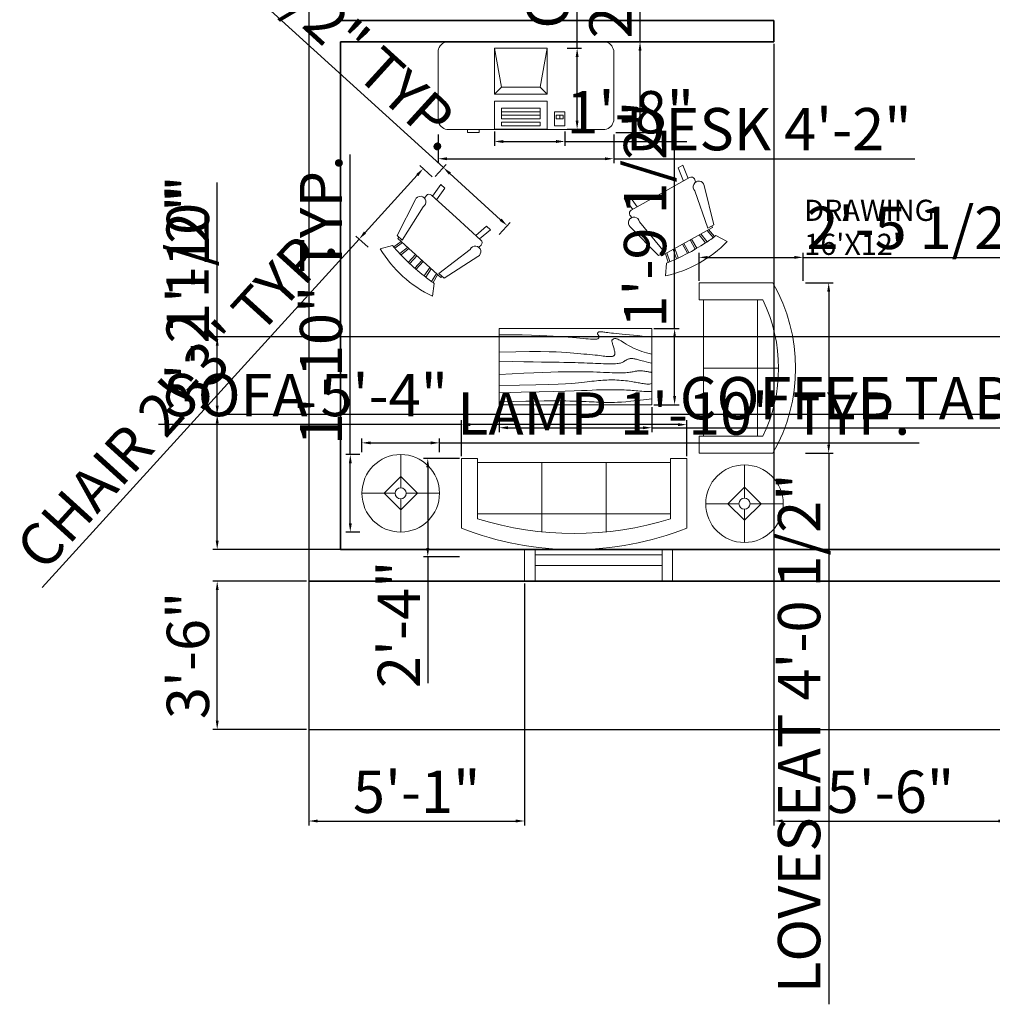
# Model space of a CAD drawing. Units: inches. Extents: x 2021 to 2692, y 429 to 1061.
# Tile 1 of 5: x 2086 to 2362, y 429 to 708. Entities that reach past the tile are written whole.
import ezdxf

# ---------------------------------------------------------------- set-up
doc = ezdxf.new("R2010")
doc.units = ezdxf.units.IN
for name, color, linetype, lineweight in [('A-ANNO-DIMS', 2, 'Continuous', 18), ('A-AREA-IDEN', 7, 'Continuous', 18), ('A-EQPM', 8, 'Continuous', 13), ('A-FURN', 8, 'Continuous', 13), ('A-GLAZ', 4, 'Continuous', 18), ('A-WALL', 7, 'Continuous', 35), ('C-PROP', 3, 'Continuous', 25)]:
    doc.layers.add(name, color=color, linetype=linetype, lineweight=lineweight)
doc.styles.get("Standard").update_dxf_attribs({"font": 'arial.ttf'})
doc.dimstyles.new('ISO-25', dxfattribs={"dimtxt": 12, "dimasz": 2.5, "dimexe": 1.25, "dimexo": 0.625, "dimtad": 1, "dimdec": 0, "dimlunit": 3, "dimtxsty": 'Standard', "dimcen": 2.5, "dimadec": 0, "dimazin": 0, "dimtfac": 1, "dimtdec": 0, "dimtmove": 0, "dimatfit": 3, "dimfxl": 1, "dimarcsym": 0})

# ---------------------------------------------------------------- blocks, each defined once
blk = doc.blocks.new('Desk - 30 x 60 in.')
for p, q in [((-26.999995, 0), (26.999995, 0)), ((-29.999995, -27), (-29.999995, -3)), ((29.999995, -3), (29.999995, -27)), ((26.999995, -30), (-26.999995, -30)), ((-20.000005, -30), (-20.000005, -31)), ((-16.000005, -31), (-16.000005, -30)), ((15.999995, -31), (15.999995, -30)), ((19.999995, -30), (19.999995, -31)), ((-20.000005, -31), (-16.000005, -31)), ((19.999995, -31), (15.999995, -31))]:
    blk.add_line(p, q)
for centre, start, end in [((-26.499995, -3.5), 98.1301, 171.8699), ((26.499995, -3.5), 8.130102, 81.8699), ((-26.499995, -26.5), 188.1301, 261.8699), ((26.499995, -26.5), 278.1301, 351.8699)]:
    blk.add_arc(centre, 3.535534, start, end)
blk = doc.blocks.new('Chair - Rocking')
for p, q in [((-8, -4.5), (-10, -1.5)), ((8, -4.5), (10, -1.5)), ((-7.5, -4.5), (-7, -7)), ((-6.5, -7), (-7.02225, -4.43)), ((-4.5, -7), (-4.96674, -4.19951)), ((-4, -7), (-4.40532, -4.16272)), ((-1.5, -4.05012), (-1.5, -7)), ((-1, -7), (-1, -4.05012)), ((1, -7), (1, -4.04655)), ((1.5, -4.05012), (1.5, -7)), ((4, -7), (4.40187, -4.18694)), ((4.5, -7), (4.96761, -4.19437)), ((6.5, -7), (7, -4.4057)), ((7.5, -4.5), (7, -7)), ((-9, -7.5), (-12, -18.49999)), ((-7, -7.5), (-9, -7.5)), ((-9, -18.49999), (-7, -7.5)), ((-8.23428, -6.99939), (-8.3093, -7.47958)), ((-8.23041, -7), (8.23915, -7)), ((7, -7.5), (9, -7.5)), ((9, -18.49999), (7, -7.5)), ((8.31071, -7.48854), (8.23449, -7.00073)), ((9, -7.5), (12, -18.49999)), ((-10.36644, -20.64523), (-10.5, -21.49999)), ((10.5, -21.49999), (10.3575, -20.58798)), ((-9, -22.49999), (-9.5, -26.49999)), ((0, -22.49999), (-9.5, -22.49999)), ((-8, -26.49999), (-7.5, -22.49999)), ((0, -22.49999), (9.5, -22.49999)), ((8, -26.49999), (7.5, -22.49999)), ((9, -22.49999), (9.5, -26.49999)), ((-9.5, -26.49999), (-8, -26.49999)), ((9.5, -26.49999), (8, -26.49999))]:
    blk.add_line(p, q)
for centre, radius, start, end in [((0, -34.08333), 34.08333, 72.93847, 107.0615), ((0, -68.25004), 64.25, 93.92211, 97.15267), ((0, -68.25004), 64.25, 82.84733, 93.92211), ((-10.5, -18.99999), 1.58114, 161.5651, 18.43495), ((10.5, -18.99999), 1.58114, 161.5651, 18.43495), ((-9.5, -21.49999), 1, 180, 270), ((9.5, -21.49999), 1, 270, 0)]:
    blk.add_arc(centre, radius, start, end)
blk = doc.blocks.new('Computer Terminal')
for p, q in [((-10, 11.5), (5, 11.5)), ((-8, 0.5), (-10, 11.5)), ((-10, -1.5), (-10, 11.5)), ((5, 11.5), (3, 0.5)), ((5, 11.5), (5, -1.5)), ((-10, -1.5), (-8, 0.5)), ((3, 0.5), (-8, 0.5)), ((3, 0.5), (5, -1.5)), ((5, -1.5), (-10, -1.5)), ((-10, -11.5), (-10, -3.5)), ((-10, -3.5), (5, -3.5)), ((-8, -5.5), (-8, -8.5)), ((3, -5.5), (-8, -5.5)), ((3, -8.5), (3, -5.5)), ((5, -3.5), (5, -11.5)), ((3, -6.5), (-8, -6.5)), ((-8, -7.5), (3, -7.5)), ((10, -6.5), (7, -6.5)), ((7, -6.5), (7, -10.5)), ((9.5, -7.5), (7.5, -7.5)), ((7.5, -7.5), (7.5, -8.5)), ((8.5, -7.5), (8.5, -8.5)), ((9.5, -8.5), (9.5, -7.5)), ((10, -10.5), (10, -6.5)), ((-8, -8.5), (3, -8.5)), ((-8, -9.5), (-8, -10.5)), ((3, -9.5), (-8, -9.5)), ((-8, -10.5), (3, -10.5)), ((3, -10.5), (3, -9.5)), ((7, -10.5), (10, -10.5)), ((7.5, -8.5), (9.5, -8.5)), ((5, -11.5), (-10, -11.5))]:
    blk.add_line(p, q)
blk = doc.blocks.new('Sofa - Roundback 7 ft.')
for p, q in [((-12.00002, -32.4421), (-12.00003, -6.5971)), ((11.99997, -32.4421), (11.99998, -6.5971)), ((-36.000027, -34), (-36.000027, -11.4696)), ((-35.999844, -13.3819), (35.9998, -13.3819)), ((35.99998, -34), (35.99998, -11.4696)), ((-36.000027, -32.4421), (35.99998, -32.4421))]:
    blk.add_line(p, q)
for points in [[(-36.000027, -34), (-42.000027, -34), (-42.000027, -8)], [(41.99998, -8), (41.99998, -34), (35.99998, -34)]]:
    blk.add_lwpolyline(points)
for centre, radius, start, end in [((0, -114.25), 114.25, 68.43141, 111.5686), ((-0.00001, -127.1968), 121.1968, 72.72033, 107.2797)]:
    blk.add_arc(centre, radius, start, end)
blk = doc.blocks.new('Sofa - Roundback Loveseat 5 ft.')
for p, q in [((0, -32.44198), (0, -5.99998)), ((-24, -33.99998), (-24, -11.46958)), ((-23.9998, -13.38178), (23.99986, -13.38178)), ((24.00004, -33.99998), (24.00004, -11.46958)), ((-24, -32.44198), (24.00004, -32.44198))]:
    blk.add_line(p, q)
for points in [[(-24, -33.99998), (-30, -33.99998), (-30, -7.99998)], [(30.00004, -7.99998), (30.00004, -33.99998), (24.00004, -33.99998)]]:
    blk.add_lwpolyline(points)
for centre, radius, start, end in [((0, -60.24998), 60.24998, 60.13715, 119.8628), ((0, -61.38438), 55.38444, 64.32083, 115.6792)]:
    blk.add_arc(centre, radius, start, end)
blk = doc.blocks.new('Table - Rectangular Woodgrain 60 x 30 in.')
for p, q in [((0, 0), (0, -30)), ((60, 0), (0, 0)), ((60, -30), (60, 0)), ((0, -30), (60, -30))]:
    blk.add_line(p, q)
for points in [[(0, -2.4), (4.8155, -2.418), (9.0302, -2.4688), (12.709, -2.5477), (15.9167, -2.65), (18.7181, -2.7711), (21.1781, -2.9063), (23.3616, -3.0508), (25.3333, -3.2), (27.1477, -3.3495), (28.8172, -3.4958), (30.3437, -3.636), (31.7291, -3.7667), (32.9756, -3.8849), (34.0849, -3.9875), (35.059, -4.0714), (35.9, -4.1334), (36.6114, -4.1711), (37.2041, -4.1854), (37.6906, -4.1779), (38.0833, -4.15), (38.3948, -4.1034), (38.6375, -4.0396), (38.8239, -3.9602), (38.9666, -3.8667), (39.0764, -3.7608), (39.1573, -3.6448), (39.2116, -3.521), (39.2416, -3.3917), (39.2498, -3.2593), (39.2385, -3.1261), (39.21, -2.9944), (39.1666, -2.8667), (39.111, -2.7447), (39.0468, -2.6281), (38.978, -2.5163), (38.9083, -2.4083), (38.8418, -2.3035), (38.7823, -2.201), (38.7337, -2.1001), (38.7, -2), (38.6844, -1.9003), (38.6875, -1.8021), (38.7094, -1.707), (38.75, -1.6167), (38.8094, -1.5326), (38.8875, -1.4563), (38.9844, -1.3893), (39.1, -1.3333), (39.2351, -1.2896), (39.3937, -1.2583), (39.5804, -1.2396), (39.8, -1.2333), (40.057, -1.2396), (40.3562, -1.2583), (40.7023, -1.2896), (41.1, -1.3333), (41.5547, -1.3895), (42.0755, -1.4573), (42.6721, -1.5361), (43.3542, -1.625), (44.1316, -1.7233), (45.014, -1.8302), (46.0114, -1.9449), (47.1333, -2.0667), (48.3862, -2.1947), (49.7625, -2.3281), (51.2513, -2.4663), (52.8416, -2.6083), (54.5226, -2.7535), (56.2833, -2.9011), (58.1127, -3.0501), (60, -3.2)], [(0, -9.2), (6.5759, -9.0858), (11.9385, -9.0365), (16.2527, -9.0418), (19.6833, -9.0917), (22.3952, -9.1759), (24.5531, -9.2844), (26.322, -9.4069), (27.8666, -9.5333), (29.3241, -9.6553), (30.7203, -9.7719), (32.0532, -9.8837), (33.3208, -9.9917), (34.5213, -10.0965), (35.6526, -10.199), (36.7128, -10.2999), (37.7, -10.4), (38.6129, -10.4996), (39.4531, -10.5969), (40.223, -10.6895), (40.925, -10.775), (41.5613, -10.8512), (42.1344, -10.9156), (42.6465, -10.966), (43.1, -11), (43.4976, -11.0158), (43.8437, -11.0136), (44.143, -10.9942), (44.4, -10.9583), (44.6195, -10.9069), (44.8062, -10.8406), (44.9648, -10.7603), (45.1, -10.6667), (45.2155, -10.5598), (45.3114, -10.4365), (45.3871, -10.2929), (45.4416, -10.125), (45.4743, -9.929), (45.4844, -9.7011), (45.4709, -9.4371), (45.4333, -9.1333), (45.3716, -8.7883), (45.2896, -8.4104), (45.1919, -8.0107), (45.0833, -7.6), (44.9685, -7.1893), (44.8521, -6.7896), (44.7388, -6.4117), (44.6333, -6.0667), (44.54, -5.7628), (44.4614, -5.4979), (44.4001, -5.2675), (44.3583, -5.0667), (44.3384, -4.8909), (44.3427, -4.7354), (44.3736, -4.5956), (44.4333, -4.4667), (44.5236, -4.3453), (44.6427, -4.2333), (44.7884, -4.1339), (44.9583, -4.05), (45.1501, -3.9849), (45.3614, -3.9417), (45.59, -3.9234), (45.8333, -3.9333), (46.0915, -3.9749), (46.3734, -4.0531), (46.6906, -4.1736), (47.0542, -4.3417), (47.4756, -4.5629), (47.9661, -4.8427), (48.5372, -5.1866), (49.2, -5.6), (49.9676, -6.0844), (50.8594, -6.625), (51.8965, -7.2031), (53.1, -7.8), (54.491, -8.3969), (56.0906, -8.975), (57.9199, -9.5156), (60, -10)], [(0, -12.8), (5.1847, -12.9322), (9.6213, -13.0323), (13.3963, -13.1059), (16.5958, -13.1583), (19.3063, -13.1952), (21.614, -13.2219), (23.6054, -13.2439), (25.3666, -13.2667), (26.9728, -13.2947), (28.4531, -13.3281), (29.8256, -13.3663), (31.1083, -13.4083), (32.3191, -13.4535), (33.476, -13.501), (34.597, -13.5501), (35.7, -13.6), (36.7984, -13.6497), (37.8875, -13.6979), (38.9578, -13.743), (40, -13.7833), (41.0047, -13.8174), (41.9625, -13.8438), (42.864, -13.8607), (43.7, -13.8667), (44.4631, -13.8604), (45.1552, -13.8417), (45.7801, -13.8104), (46.3416, -13.7667), (46.8439, -13.7104), (47.2906, -13.6417), (47.6858, -13.5604), (48.0333, -13.4667), (48.3375, -13.3608), (48.6042, -13.2448), (48.8396, -13.121), (49.05, -12.9917), (49.2417, -12.8593), (49.4208, -12.7261), (49.5937, -12.5944), (49.7667, -12.4667), (49.9452, -12.3451), (50.1323, -12.2313), (50.3303, -12.1268), (50.5416, -12.0333), (50.7686, -11.9524), (51.0135, -11.8854), (51.2788, -11.8341), (51.5666, -11.8), (51.8785, -11.7843), (52.2116, -11.7865), (52.562, -11.8059), (52.926, -11.8417), (53.2998, -11.8931), (53.6795, -11.9594), (54.0614, -12.0397), (54.4416, -12.1333), (54.8223, -12.2401), (55.2293, -12.3625), (55.6942, -12.5037), (56.2489, -12.6667), (56.9251, -12.8547), (57.7545, -13.0708), (58.7689, -13.3182), (60, -13.6)], [(0, -18), (5.124, -17.7273), (9.6609, -17.5057), (13.6705, -17.3303), (17.2125, -17.1958), (20.3467, -17.0973), (23.1328, -17.0297), (25.6307, -16.9878), (27.9, -16.9667), (29.9928, -16.9617), (31.9302, -16.9703), (33.7254, -16.9907), (35.3917, -17.0208), (36.9423, -17.0588), (38.3906, -17.1026), (39.7499, -17.1503), (41.0333, -17.2), (42.2519, -17.2496), (43.4073, -17.2969), (44.4986, -17.3395), (45.525, -17.375), (46.4858, -17.4012), (47.3802, -17.4156), (48.2074, -17.416), (48.9667, -17.4), (49.6583, -17.3662), (50.2872, -17.3167), (50.8595, -17.2547), (51.3812, -17.1833), (51.8584, -17.1057), (52.2971, -17.025), (52.7034, -16.9443), (53.0833, -16.8667), (53.443, -16.7951), (53.789, -16.7313), (54.128, -16.6768), (54.4666, -16.6334), (54.8115, -16.6024), (55.1693, -16.5854), (55.5465, -16.5841), (55.95, -16.6), (56.3828, -16.6337), (56.8346, -16.6823), (57.2915, -16.7418), (57.7396, -16.8084), (58.165, -16.878), (58.5539, -16.9469), (58.8924, -17.0111), (59.1666, -17.0667), (59.3679, -17.1107), (59.5078, -17.1438), (59.6032, -17.1675), (59.6708, -17.1833), (59.7275, -17.193), (59.7901, -17.1979), (59.8753, -17.1998), (60, -17.2)], [(0, -22.4), (8.0098, -22.2501), (14.4094, -22.1011), (19.4168, -21.9535), (23.25, -21.8083), (26.1269, -21.6663), (28.2656, -21.5281), (29.884, -21.3947), (31.2, -21.2667), (32.3967, -21.1448), (33.5172, -21.0292), (34.5697, -20.9198), (35.5625, -20.8167), (36.5037, -20.7198), (37.4015, -20.6292), (38.2642, -20.5448), (39.1, -20.4667), (39.9164, -20.3951), (40.7187, -20.3313), (41.5117, -20.2768), (42.3, -20.2333), (43.0883, -20.2024), (43.8812, -20.1854), (44.6836, -20.1841), (45.5, -20.2), (46.3328, -20.234), (47.1747, -20.2844), (48.0163, -20.3488), (48.8479, -20.425), (49.66, -20.5106), (50.4429, -20.6031), (51.1872, -20.7004), (51.8833, -20.8), (52.5246, -20.8999), (53.1166, -20.9995), (53.6681, -21.0983), (54.1875, -21.1958), (54.6834, -21.2919), (55.1646, -21.3859), (55.6394, -21.4777), (56.1167, -21.5667), (56.6028, -21.6515), (57.0961, -21.7266), (57.5929, -21.7852), (58.0896, -21.8208), (58.5823, -21.8268), (59.0674, -21.7964), (59.5412, -21.723), (60, -21.6)], [(0, -25.2), (8.6355, -25.0504), (15.7026, -24.9031), (21.4049, -24.7606), (25.9458, -24.625), (29.529, -24.4988), (32.3578, -24.3844), (34.6359, -24.284), (36.5667, -24.2), (38.3213, -24.1341), (39.9417, -24.0854), (41.437, -24.0523), (42.8167, -24.0333), (44.0901, -24.0268), (45.2667, -24.0313), (46.3557, -24.0451), (47.3667, -24.0667), (48.309, -24.0947), (49.1928, -24.1287), (50.0284, -24.168), (50.826, -24.2125), (51.5959, -24.2617), (52.3483, -24.3151), (53.0935, -24.3725), (53.8417, -24.4334), (54.6009, -24.497), (55.3699, -24.561), (56.1454, -24.6226), (56.9239, -24.6792), (57.7021, -24.7279), (58.4764, -24.7662), (59.2435, -24.7911), (60, -24.8)], [(0, -28.8), (5.6867, -28.6681), (10.45, -28.5698), (14.407, -28.5012), (17.675, -28.4584), (20.3711, -28.4374), (22.6125, -28.4344), (24.5164, -28.4455), (26.2, -28.4667), (27.762, -28.4947), (29.2276, -28.5281), (30.6033, -28.5663), (31.8958, -28.6084), (33.1118, -28.6535), (34.2578, -28.7011), (35.3405, -28.7501), (36.3666, -28.8), (37.3443, -28.8497), (38.288, -28.8974), (39.2137, -28.9412), (40.1375, -28.9792), (41.0753, -29.0093), (42.0432, -29.0297), (43.0572, -29.0384), (44.1333, -29.0333), (45.2936, -29.0114), (46.5843, -28.9641), (48.0579, -28.8816), (49.7666, -28.7542), (51.7629, -28.5721), (54.0989, -28.3255), (56.8272, -28.0048), (60, -27.6)]]:
    blk.add_lwpolyline(points)
blk = doc.blocks.new('Lamp - Table')
for p, q in [((0, 7), (0, 1)), ((0, 3), (-3, 0)), ((3, 0), (0, 3)), ((-1, 0), (-7, 0)), ((-3, 0), (0, -3)), ((0, -3), (3, 0)), ((1, 0), (7, 0)), ((0, -1), (0, -7))]:
    blk.add_line(p, q)
for radius in [7, 1]:
    blk.add_circle((0, 0), radius)
blk = doc.blocks.new('WIN-36IN')
for p, q in [((0, 0), (0, 9)), ((3, 9), (39, 9)), ((3, 0), (3, 9)), ((39, 9), (39, 0)), ((42, 9), (42, 0)), ((3, 7.5), (39, 7.5)), ((3, 4.5), (39, 4.5)), ((39, 0), (3, 0))]:
    blk.add_line(p, q)
blk = doc.blocks.new('*D22')
at = {"layer": 'A-ANNO-DIMS', "color": 0, "lineweight": -2, "transparency": 16777216}
for p, q in [((2203.07, 663.69), (2199.61, 666.84)), ((2198.85, 664.15), (2184.05, 647.87)), ((2182.37, 646.02), (2092.52, 547.18)), ((2184.9, 643.71), (2181.45, 646.86))]:
    blk.add_line(p, q, dxfattribs=at)
at = {"layer": 'A-ANNO-DIMS', "color": 0, "transparency": 16777216}
for points in [[(2198.54, 664.43), (2199.16, 663.87), (2200.53, 666)], [(2183.74, 648.15), (2184.36, 647.59), (2182.37, 646.02)]]:
    blk.add_solid(points, dxfattribs=at)
at = {"layer": 'Defpoints', "color": 0, "transparency": 16777216}
for p in [(2203.53, 663.27), (2182.37, 646.02), (2185.37, 643.29)]:
    blk.add_point(p, dxfattribs=at)
at = {"layer": 'A-ANNO-DIMS', "color": 0, "transparency": 16777216, "insert": (2131.55, 600.27), "char_height": 12, "attachment_point": 5, "rotation": 47.7243}
blk.add_mtext('CHAIR 2\'-3" TYP.', dxfattribs=at)
blk = doc.blocks.new('*D23')
at = {"layer": 'A-ANNO-DIMS', "color": 0, "lineweight": -2, "transparency": 16777216}
for p, q in [((2206.25, 666.27), (2128.52, 736.94)), ((2203.95, 663.73), (2207.09, 667.19)), ((2222.48, 651.51), (2208.1, 664.59)), ((2222.03, 647.3), (2225.17, 650.75))]:
    blk.add_line(p, q, dxfattribs=at)
at = {"layer": 'A-ANNO-DIMS', "color": 0, "transparency": 16777216}
for points in [[(2208.38, 664.89), (2207.82, 664.28), (2206.25, 666.27)], [(2222.76, 651.82), (2222.2, 651.2), (2224.33, 649.83)]]:
    blk.add_solid(points, dxfattribs=at)
at = {"layer": 'Defpoints', "color": 0, "transparency": 16777216}
for p in [(2206.25, 666.27), (2203.53, 663.27), (2221.61, 646.83)]:
    blk.add_point(p, dxfattribs=at)
at = {"layer": 'A-ANNO-DIMS', "color": 0, "transparency": 16777216, "insert": (2171.05, 707.5), "char_height": 12, "attachment_point": 5, "rotation": 317.7243}
blk.add_mtext('2\'-0 1/2" TYP.', dxfattribs=at)
blk = doc.blocks.new('*D24')
at = {"layer": 'A-ANNO-DIMS', "color": 0, "lineweight": -2, "transparency": 16777216}
for p, q in [((2183.16, 585.54), (2183.16, 589.47)), ((2205.16, 585.54), (2205.16, 589.47)), ((2185.66, 588.22), (2202.66, 588.22)), ((2205.16, 588.22), (2341.16, 588.22))]:
    blk.add_line(p, q, dxfattribs=at)
at = {"layer": 'A-ANNO-DIMS', "color": 0, "transparency": 16777216}
for points in [[(2185.66, 588.63), (2185.66, 587.8), (2183.16, 588.22)], [(2202.66, 588.63), (2202.66, 587.8), (2205.16, 588.22)]]:
    blk.add_solid(points, dxfattribs=at)
at = {"layer": 'Defpoints', "color": 0, "transparency": 16777216}
for p in [(2205.16, 588.22), (2183.16, 584.92), (2205.16, 584.92)]:
    blk.add_point(p, dxfattribs=at)
at = {"layer": 'A-ANNO-DIMS', "color": 0, "transparency": 16777216, "insert": (2274.41, 594.97), "char_height": 12, "attachment_point": 5}
blk.add_mtext('LAMP 1\'-10" TYP.', dxfattribs=at)
blk = doc.blocks.new('*D25')
at = {"layer": 'A-ANNO-DIMS', "color": 0, "lineweight": -2, "transparency": 16777216}
for p, q in [((2179.86, 584.92), (2179.86, 670.01)), ((2182.54, 584.92), (2178.61, 584.92)), ((2179.86, 565.42), (2179.86, 582.42)), ((2182.54, 562.92), (2178.61, 562.92))]:
    blk.add_line(p, q, dxfattribs=at)
at = {"layer": 'A-ANNO-DIMS', "color": 0, "transparency": 16777216}
for points in [[(2179.45, 582.42), (2180.28, 582.42), (2179.86, 584.92)], [(2179.45, 565.42), (2180.28, 565.42), (2179.86, 562.92)]]:
    blk.add_solid(points, dxfattribs=at)
at = {"layer": 'Defpoints', "color": 0, "transparency": 16777216}
for p in [(2179.86, 584.92), (2183.16, 584.92), (2183.16, 562.92)]:
    blk.add_point(p, dxfattribs=at)
at = {"layer": 'A-ANNO-DIMS', "color": 0, "transparency": 16777216, "insert": (2173.11, 628.71), "char_height": 12, "attachment_point": 5, "rotation": 90}
blk.add_mtext('1\'-10" TYP.', dxfattribs=at)
blk = doc.blocks.new('*D40')
at = {"layer": 'A-ANNO-DIMS', "color": 0, "lineweight": -2, "transparency": 16777216}
for p, q in [((2204.78, 675.63), (2204.78, 667.54)), ((2254.55, 675.63), (2254.55, 667.54)), ((2207.28, 668.79), (2252.05, 668.79)), ((2254.55, 668.79), (2339.91, 668.79))]:
    blk.add_line(p, q, dxfattribs=at)
at = {"layer": 'A-ANNO-DIMS', "color": 0, "transparency": 16777216}
for points in [[(2207.28, 669.2), (2207.28, 668.37), (2204.78, 668.79)], [(2252.05, 669.2), (2252.05, 668.37), (2254.55, 668.79)]]:
    blk.add_solid(points, dxfattribs=at)
at = {"layer": 'Defpoints', "color": 0, "transparency": 16777216}
for p in [(2204.78, 676.25), (2254.55, 676.25), (2254.55, 668.79)]:
    blk.add_point(p, dxfattribs=at)
at = {"layer": 'A-ANNO-DIMS', "color": 0, "transparency": 16777216, "insert": (2298.48, 675.62), "char_height": 12, "attachment_point": 5}
blk.add_mtext('DESK 4\'-2"', dxfattribs=at)
blk = doc.blocks.new('*D41')
at = {"layer": 'A-ANNO-DIMS', "color": 0, "lineweight": -2, "transparency": 16777216}
for p, q in [((2262.01, 701.96), (2262.01, 765.78)), ((2255.17, 701.96), (2263.26, 701.96)), ((2262.01, 678.75), (2262.01, 699.46)), ((2255.17, 676.25), (2263.26, 676.25))]:
    blk.add_line(p, q, dxfattribs=at)
at = {"layer": 'A-ANNO-DIMS', "color": 0, "transparency": 16777216}
for points in [[(2261.6, 699.46), (2262.43, 699.46), (2262.01, 701.96)], [(2261.6, 678.75), (2262.43, 678.75), (2262.01, 676.25)]]:
    blk.add_solid(points, dxfattribs=at)
at = {"layer": 'Defpoints', "color": 0, "transparency": 16777216}
for p in [(2254.55, 701.96), (2262.01, 701.96), (2254.55, 676.25)]:
    blk.add_point(p, dxfattribs=at)
at = {"layer": 'A-ANNO-DIMS', "color": 0, "transparency": 16777216, "insert": (2255.18, 735.12), "char_height": 12, "attachment_point": 5, "rotation": 90}
blk.add_mtext('2\'-1 1/2"', dxfattribs=at)
blk = doc.blocks.new('*D42')
at = {"layer": 'A-ANNO-DIMS', "color": 0, "lineweight": -2, "transparency": 16777216}
for p, q in [((2244.18, 700.13), (2244.18, 845.55)), ((2241.36, 700.13), (2245.43, 700.13)), ((2244.18, 679.63), (2244.18, 697.63)), ((2241.36, 677.13), (2245.43, 677.13))]:
    blk.add_line(p, q, dxfattribs=at)
at = {"layer": 'A-ANNO-DIMS', "color": 0, "transparency": 16777216}
for points in [[(2243.76, 697.63), (2244.6, 697.63), (2244.18, 700.13)], [(2243.76, 679.63), (2244.6, 679.63), (2244.18, 677.13)]]:
    blk.add_solid(points, dxfattribs=at)
at = {"layer": 'Defpoints', "color": 0, "transparency": 16777216}
for p in [(2240.73, 700.13), (2244.18, 700.13), (2240.73, 677.13)]:
    blk.add_point(p, dxfattribs=at)
at = {"layer": 'A-ANNO-DIMS', "color": 0, "transparency": 16777216, "insert": (2237.35, 774.09), "char_height": 12, "attachment_point": 5, "rotation": 90}
blk.add_mtext('COMPUTER 1\'-11"', dxfattribs=at)
blk = doc.blocks.new('*D43')
at = {"layer": 'A-ANNO-DIMS', "color": 0, "lineweight": -2, "transparency": 16777216}
for p, q in [((2220.73, 676.5), (2220.73, 672.43)), ((2240.73, 676.5), (2240.73, 672.43)), ((2223.23, 673.68), (2238.23, 673.68)), ((2240.73, 673.68), (2275.25, 673.68))]:
    blk.add_line(p, q, dxfattribs=at)
at = {"layer": 'A-ANNO-DIMS', "color": 0, "transparency": 16777216}
for points in [[(2223.23, 674.09), (2223.23, 673.26), (2220.73, 673.68)], [(2238.23, 674.09), (2238.23, 673.26), (2240.73, 673.68)]]:
    blk.add_solid(points, dxfattribs=at)
at = {"layer": 'Defpoints', "color": 0, "transparency": 16777216}
for p in [(2220.73, 677.13), (2240.73, 677.13), (2240.73, 673.68)]:
    blk.add_point(p, dxfattribs=at)
at = {"layer": 'A-ANNO-DIMS', "color": 0, "transparency": 16777216, "insert": (2259.24, 680.43), "char_height": 12, "attachment_point": 5}
blk.add_mtext('1\'-8"', dxfattribs=at)
blk = doc.blocks.new('*D44')
at = {"layer": 'A-ANNO-DIMS', "color": 0, "lineweight": -2, "transparency": 16777216}
for p, q in [((2211.41, 593.39), (2125.52, 593.39)), ((2211.41, 584.43), (2211.41, 594.64)), ((2272.76, 593.39), (2213.91, 593.39)), ((2275.26, 584.43), (2275.26, 594.64))]:
    blk.add_line(p, q, dxfattribs=at)
at = {"layer": 'A-ANNO-DIMS', "color": 0, "transparency": 16777216}
for points in [[(2213.91, 593.8), (2213.91, 592.97), (2211.41, 593.39)], [(2272.76, 593.8), (2272.76, 592.97), (2275.26, 593.39)]]:
    blk.add_solid(points, dxfattribs=at)
at = {"layer": 'Defpoints', "color": 0, "transparency": 16777216}
for p in [(2211.41, 593.39), (2211.41, 583.81), (2275.26, 583.81)]:
    blk.add_point(p, dxfattribs=at)
at = {"layer": 'A-ANNO-DIMS', "color": 0, "transparency": 16777216, "insert": (2167.21, 600.22), "char_height": 12, "attachment_point": 5}
blk.add_mtext('SOFA 5\'-4"', dxfattribs=at)
blk = doc.blocks.new('*D45')
at = {"layer": 'A-ANNO-DIMS', "color": 0, "lineweight": -2, "transparency": 16777216}
for p, q in [((2210.78, 583.81), (2200.58, 583.81)), ((2201.83, 581.31), (2201.83, 558.44)), ((2210.78, 555.94), (2200.58, 555.94)), ((2201.83, 555.94), (2201.83, 520.08))]:
    blk.add_line(p, q, dxfattribs=at)
at = {"layer": 'A-ANNO-DIMS', "color": 0, "transparency": 16777216}
for points in [[(2201.41, 581.31), (2202.25, 581.31), (2201.83, 583.81)], [(2201.41, 558.44), (2202.25, 558.44), (2201.83, 555.94)]]:
    blk.add_solid(points, dxfattribs=at)
at = {"layer": 'Defpoints', "color": 0, "transparency": 16777216}
for p in [(2211.41, 583.81), (2201.83, 555.94), (2211.41, 555.94)]:
    blk.add_point(p, dxfattribs=at)
at = {"layer": 'A-ANNO-DIMS', "color": 0, "transparency": 16777216, "insert": (2195.18, 536.76), "char_height": 12, "attachment_point": 5, "rotation": 90}
blk.add_mtext('2\'-4"', dxfattribs=at)
blk = doc.blocks.new('*D46')
at = {"layer": 'A-ANNO-DIMS', "color": 0, "lineweight": -2, "transparency": 16777216}
for p, q in [((2308.89, 633.57), (2316.76, 633.57)), ((2315.51, 631.07), (2315.51, 587.75)), ((2308.89, 585.25), (2316.76, 585.25)), ((2315.51, 585.25), (2315.51, 429))]:
    blk.add_line(p, q, dxfattribs=at)
at = {"layer": 'A-ANNO-DIMS', "color": 0, "transparency": 16777216}
for points in [[(2315.1, 631.07), (2315.93, 631.07), (2315.51, 633.57)], [(2315.1, 587.75), (2315.93, 587.75), (2315.51, 585.25)]]:
    blk.add_solid(points, dxfattribs=at)
at = {"layer": 'Defpoints', "color": 0, "transparency": 16777216}
for p in [(2308.26, 633.57), (2308.26, 585.25), (2315.51, 585.25)]:
    blk.add_point(p, dxfattribs=at)
at = {"layer": 'A-ANNO-DIMS', "color": 0, "transparency": 16777216, "insert": (2308.68, 505.87), "char_height": 12, "attachment_point": 5, "rotation": 90}
blk.add_mtext('LOVESEAT 4\'-0 1/2"', dxfattribs=at)
blk = doc.blocks.new('*D47')
at = {"layer": 'A-ANNO-DIMS', "color": 0, "lineweight": -2, "transparency": 16777216}
for p, q in [((2278.74, 634.19), (2278.74, 642.06)), ((2281.24, 640.81), (2305.76, 640.81)), ((2308.26, 634.19), (2308.26, 642.06)), ((2308.26, 640.81), (2372.08, 640.81))]:
    blk.add_line(p, q, dxfattribs=at)
at = {"layer": 'A-ANNO-DIMS', "color": 0, "transparency": 16777216}
for points in [[(2281.24, 641.23), (2281.24, 640.4), (2278.74, 640.81)], [(2305.76, 641.23), (2305.76, 640.4), (2308.26, 640.81)]]:
    blk.add_solid(points, dxfattribs=at)
at = {"layer": 'Defpoints', "color": 0, "transparency": 16777216}
for p in [(2308.26, 640.81), (2278.74, 633.57), (2308.26, 633.57)]:
    blk.add_point(p, dxfattribs=at)
at = {"layer": 'A-ANNO-DIMS', "color": 0, "transparency": 16777216, "insert": (2341.42, 647.64), "char_height": 12, "attachment_point": 5}
blk.add_mtext('2\'-5 1/2"', dxfattribs=at)
blk = doc.blocks.new('*D48')
at = {"layer": 'A-ANNO-DIMS', "color": 0, "lineweight": -2, "transparency": 16777216}
for p, q in [((2222.09, 598.36), (2222.09, 591.25)), ((2265.33, 598.36), (2265.33, 591.25)), ((2224.59, 592.5), (2262.83, 592.5)), ((2265.33, 592.5), (2431.25, 592.5))]:
    blk.add_line(p, q, dxfattribs=at)
at = {"layer": 'A-ANNO-DIMS', "color": 0, "transparency": 16777216}
for points in [[(2224.59, 592.92), (2224.59, 592.08), (2222.09, 592.5)], [(2262.83, 592.92), (2262.83, 592.08), (2265.33, 592.5)]]:
    blk.add_solid(points, dxfattribs=at)
at = {"layer": 'Defpoints', "color": 0, "transparency": 16777216}
for p in [(2222.09, 598.99), (2265.33, 598.99), (2265.33, 592.5)]:
    blk.add_point(p, dxfattribs=at)
at = {"layer": 'A-ANNO-DIMS', "color": 0, "transparency": 16777216, "insert": (2349.54, 599.34), "char_height": 12, "attachment_point": 5}
blk.add_mtext('COFFEE TABLE 3\'-7"', dxfattribs=at)
blk = doc.blocks.new('*D49')
at = {"layer": 'A-ANNO-DIMS', "color": 0, "lineweight": -2, "transparency": 16777216}
for p, q in [((2271.82, 620.61), (2271.82, 683.09)), ((2265.96, 620.61), (2273.07, 620.61)), ((2271.82, 601.49), (2271.82, 618.11)), ((2265.96, 598.99), (2273.07, 598.99))]:
    blk.add_line(p, q, dxfattribs=at)
at = {"layer": 'A-ANNO-DIMS', "color": 0, "transparency": 16777216}
for points in [[(2271.4, 618.11), (2272.23, 618.11), (2271.82, 620.61)], [(2271.4, 601.49), (2272.23, 601.49), (2271.82, 598.99)]]:
    blk.add_solid(points, dxfattribs=at)
at = {"layer": 'Defpoints', "color": 0, "transparency": 16777216}
for p in [(2265.33, 620.61), (2271.82, 620.61), (2265.33, 598.99)]:
    blk.add_point(p, dxfattribs=at)
at = {"layer": 'A-ANNO-DIMS', "color": 0, "transparency": 16777216, "insert": (2264.99, 653.1), "char_height": 12, "attachment_point": 5, "rotation": 90}
blk.add_mtext('1\'-9 1/2"', dxfattribs=at)
blk = doc.blocks.new('*D54')
at = {"layer": 'A-ANNO-DIMS', "color": 0, "lineweight": -2, "transparency": 16777216}
for p, q in [((2167.48, 548.96), (2140.87, 548.96)), ((2142.12, 509.46), (2142.12, 546.46)), ((2167.48, 506.96), (2140.87, 506.96))]:
    blk.add_line(p, q, dxfattribs=at)
at = {"layer": 'A-ANNO-DIMS', "color": 0, "transparency": 16777216}
for points in [[(2141.71, 546.46), (2142.54, 546.46), (2142.12, 548.96)], [(2141.71, 509.46), (2142.54, 509.46), (2142.12, 506.96)]]:
    blk.add_solid(points, dxfattribs=at)
at = {"layer": 'Defpoints', "color": 0, "transparency": 16777216}
for p in [(2142.12, 548.96), (2168.11, 548.96), (2168.11, 506.96)]:
    blk.add_point(p, dxfattribs=at)
at = {"layer": 'A-ANNO-DIMS', "color": 0, "transparency": 16777216, "insert": (2135.37, 527.96), "char_height": 12, "attachment_point": 5, "rotation": 90}
blk.add_mtext('3\'-6"', dxfattribs=at)
blk = doc.blocks.new('*D62')
at = {"layer": 'A-ANNO-DIMS', "color": 0, "lineweight": -2, "transparency": 16777216}
for p, q in [((2168.11, 548.34), (2168.11, 479.73)), ((2229.27, 548.34), (2229.27, 479.73)), ((2170.61, 480.98), (2226.77, 480.98))]:
    blk.add_line(p, q, dxfattribs=at)
at = {"layer": 'A-ANNO-DIMS', "color": 0, "transparency": 16777216}
for points in [[(2170.61, 481.4), (2170.61, 480.56), (2168.11, 480.98)], [(2226.77, 481.4), (2226.77, 480.56), (2229.27, 480.98)]]:
    blk.add_solid(points, dxfattribs=at)
at = {"layer": 'Defpoints', "color": 0, "transparency": 16777216}
for p in [(2168.11, 548.96), (2229.27, 548.96), (2229.27, 480.98)]:
    blk.add_point(p, dxfattribs=at)
at = {"layer": 'A-ANNO-DIMS', "color": 0, "transparency": 16777216, "insert": (2198.69, 487.73), "char_height": 12, "attachment_point": 5}
blk.add_mtext('5\'-1"', dxfattribs=at)
blk = doc.blocks.new('*D68')
at = {"layer": 'A-ANNO-DIMS', "color": 0, "lineweight": -2, "transparency": 16777216}
for p, q in [((2299.94, 701.34), (2299.94, 479.73)), ((2366.11, 701.34), (2366.11, 479.73)), ((2302.44, 480.98), (2363.61, 480.98))]:
    blk.add_line(p, q, dxfattribs=at)
at = {"layer": 'A-ANNO-DIMS', "color": 0, "transparency": 16777216}
for points in [[(2302.44, 481.4), (2302.44, 480.56), (2299.94, 480.98)], [(2363.61, 481.4), (2363.61, 480.56), (2366.11, 480.98)]]:
    blk.add_solid(points, dxfattribs=at)
at = {"layer": 'Defpoints', "color": 0, "transparency": 16777216}
for p in [(2299.94, 701.96), (2366.11, 701.96), (2366.11, 480.98)]:
    blk.add_point(p, dxfattribs=at)
at = {"layer": 'A-ANNO-DIMS', "color": 0, "transparency": 16777216, "insert": (2333.02, 487.73), "char_height": 12, "attachment_point": 5}
blk.add_mtext('5\'-6"', dxfattribs=at)
blk = doc.blocks.new('*D69')
at = {"layer": 'A-ANNO-DIMS', "color": 0, "lineweight": -2, "transparency": 16777216}
for p, q in [((2142.12, 596.25), (2142.12, 659.85)), ((2368.48, 596.25), (2140.87, 596.25)), ((2142.12, 560.46), (2142.12, 593.75)), ((2368.48, 557.96), (2140.87, 557.96))]:
    blk.add_line(p, q, dxfattribs=at)
at = {"layer": 'A-ANNO-DIMS', "color": 0, "transparency": 16777216}
for points in [[(2141.71, 593.75), (2142.54, 593.75), (2142.12, 596.25)], [(2141.71, 560.46), (2142.54, 560.46), (2142.12, 557.96)]]:
    blk.add_solid(points, dxfattribs=at)
at = {"layer": 'Defpoints', "color": 0, "transparency": 16777216}
for p in [(2142.12, 596.25), (2369.11, 596.25), (2369.11, 557.96)]:
    blk.add_point(p, dxfattribs=at)
at = {"layer": 'A-ANNO-DIMS', "color": 0, "transparency": 16777216, "insert": (2135.29, 629.3), "char_height": 12, "attachment_point": 5, "rotation": 90}
blk.add_mtext('3\'-2 1/2"', dxfattribs=at)
blk = doc.blocks.new('*D70')
at = {"layer": 'A-ANNO-DIMS', "color": 0, "lineweight": -2, "transparency": 16777216}
for p, q in [((2142.12, 618.25), (2142.12, 662.09)), ((2368.48, 618.25), (2140.87, 618.25)), ((2142.12, 598.75), (2142.12, 615.75)), ((2368.48, 596.25), (2140.87, 596.25))]:
    blk.add_line(p, q, dxfattribs=at)
at = {"layer": 'A-ANNO-DIMS', "color": 0, "transparency": 16777216}
for points in [[(2141.71, 615.75), (2142.54, 615.75), (2142.12, 618.25)], [(2141.71, 598.75), (2142.54, 598.75), (2142.12, 596.25)]]:
    blk.add_solid(points, dxfattribs=at)
at = {"layer": 'Defpoints', "color": 0, "transparency": 16777216}
for p in [(2142.12, 618.25), (2369.11, 618.25), (2369.11, 596.25)]:
    blk.add_point(p, dxfattribs=at)
at = {"layer": 'A-ANNO-DIMS', "color": 0, "transparency": 16777216, "insert": (2135.37, 641.42), "char_height": 12, "attachment_point": 5, "rotation": 90}
blk.add_mtext('1\'-10"', dxfattribs=at)

msp = doc.modelspace()

# ---------------------------------------------------------------- linework, layer by layer
at = {"layer": 'A-WALL'}
for p, q in [((2177.11, 827.96), (2177.11, 707.96)), ((2299.94, 707.96), (2177.11, 707.96)), ((2299.94, 707.96), (2299.94, 701.96)), ((2177.11, 701.96), (2177.11, 557.96)), ((2299.94, 701.96), (2177.11, 701.96)), ((2369.11, 557.96), (2177.11, 557.96)), ((2369.11, 548.96), (2168.11, 548.96))]:
    msp.add_line(p, q, dxfattribs=at)
at = {"layer": 'C-PROP'}
msp.add_lwpolyline([(2168.11, 506.96), (2528.11, 506.96), (2528.11, 986.96), (2168.11, 986.96)], close=True, dxfattribs=at)

# ---------------------------------------------------------------- block references
at = {"layer": 'A-EQPM'}
msp.add_blockref('Computer Terminal', (2230.73, 688.63), dxfattribs=at)
at = {"layer": 'A-FURN'}
for name, p, xscale, yscale, zscale in [('Desk - 30 x 60 in.', (2229.66, 701.96), 0.8294180658732822, 0.8294180658732822, 0.8294180658732822), ('Table - Rectangular Woodgrain 60 x 30 in.', (2222.09, 620.61), 0.7206596845232396, 0.7206596845232396, 0.7206596845232396), ('Lamp - Table', (2194.16, 573.92), 1.571428663265289, 1.571428663265289, 1.571428663265289), ('Lamp - Table', (2291.63, 570.97), 1.571428663265289, 1.571428663265289, 1.571428663265289)]:
    msp.add_blockref(name, p, dxfattribs=dict(at, xscale=xscale, yscale=yscale, zscale=zscale))
for p, rotation in [((2278.74, 639.16), 209.1183388143818), ((2194.74, 635.44), 137.7242525859534)]:
    msp.add_blockref('Chair - Rocking', p, dxfattribs=dict(at, rotation=rotation))
for name, p, xscale, yscale, zscale, rotation in [('Sofa - Roundback Loveseat 5 ft.', (2306.12, 609.41), 0.8053303952886803, 0.8053303952886803, 0.8053303952886803, 270), ('Sofa - Roundback 7 ft.', (2243.33, 557.96), 0.7601400613229315, 0.7601400613229315, 0.7601400613229315, 180)]:
    msp.add_blockref(name, p, dxfattribs=dict(at, xscale=xscale, yscale=yscale, zscale=zscale, rotation=rotation))
at = {"layer": 'A-GLAZ'}
msp.add_blockref('WIN-36IN', (2229.27, 548.96), dxfattribs=at)

# ---------------------------------------------------------------- texts
at = {"layer": 'A-AREA-IDEN'}
for s, p in [('DRAWING', (2308.57, 651.16)), ("16'X12'", (2308.57, 641.52))]:
    msp.add_text(s, height=6, dxfattribs=at).set_placement(p)

# ---------------------------------------------------------------- dimensions: what is measured, and where the dimension line sits
at = {"layer": 'A-ANNO-DIMS'}
for base, p1, p2, angle, text, picture, middle in [((2244.18, 700.13), (2240.73, 677.13), (2240.73, 700.13), 90, 'COMPUTER <>', '*D42', (2237.35, 774.09)), ((2206.25, 666.27), (2221.61, 646.83), (2203.53, 663.27), 137.7243, '<> TYP.', '*D23', (2171.05, 707.5)), ((2179.86, 584.92), (2183.16, 562.92), (2183.16, 584.92), 90, '<> TYP.', '*D25', (2173.11, 628.71)), ((2182.37, 646.02), (2203.53, 663.27), (2185.37, 643.29), 227.7243, 'CHAIR <> TYP.', '*D22', (2131.55, 600.27)), ((2315.51, 585.25), (2308.26, 633.57), (2308.26, 585.25), 270, 'LOVESEAT <>', '*D46', (2308.68, 505.87)), ((2211.4081, 593.3868), (2275.2598, 583.809), (2211.4081, 583.809), 180, 'SOFA <>', '*D44', (2167.2121, 600.2205))]:
    dim = msp.add_linear_dim(base=base, p1=p1, p2=p2, angle=angle, text=text, dimstyle='ISO-25', override={"dimdec": 1, "dimlfac": 1, "dimrnd": 0, "dimzin": 1, "dimdsep": 46, "dimlunit": 4, "dimfrac": 2}, dxfattribs=at)
    dim.commit()
    dim.dimension.update_dxf_attribs({"geometry": picture, "text_midpoint": middle})
for base, p1, p2, angle, picture, middle in [((2262.01, 701.96), (2254.55, 676.25), (2254.55, 701.96), 90, '*D41', (2255.18, 735.12)), ((2271.82, 620.61), (2265.33, 598.99), (2265.33, 620.61), 90, '*D49', (2264.99, 653.1)), ((2142.12, 618.25), (2369.11, 596.25), (2369.11, 618.25), 90, '*D70', (2135.37, 641.42)), ((2142.12, 596.25), (2369.11, 557.96), (2369.11, 596.25), 90, '*D69', (2135.29, 629.3)), ((2201.83, 555.94), (2211.41, 583.81), (2211.41, 555.94), 270, '*D45', (2195.18, 536.76)), ((2142.12, 548.96), (2168.11, 506.96), (2168.11, 548.96), 90, '*D54', (2135.37, 527.96))]:
    dim = msp.add_linear_dim(base=base, p1=p1, p2=p2, angle=angle, dimstyle='ISO-25', override={"dimdec": 1, "dimlfac": 1, "dimrnd": 0, "dimzin": 1, "dimdsep": 46, "dimlunit": 4, "dimfrac": 2}, dxfattribs=at)
    dim.commit()
    dim.dimension.update_dxf_attribs({"geometry": picture, "text_midpoint": middle})
for base, p1, p2, picture, middle in [((2366.11, 480.98), (2299.94, 701.96), (2366.11, 701.96), '*D68', (2333.02, 487.73)), ((2240.73, 673.68), (2220.73, 677.13), (2240.73, 677.13), '*D43', (2259.24, 680.43)), ((2308.26, 640.81), (2278.74, 633.57), (2308.26, 633.57), '*D47', (2341.42, 647.64)), ((2229.27, 480.98), (2168.11, 548.96), (2229.27, 548.96), '*D62', (2198.69, 487.73))]:
    dim = msp.add_linear_dim(base=base, p1=p1, p2=p2, dimstyle='ISO-25', override={"dimdec": 1, "dimlfac": 1, "dimrnd": 0, "dimzin": 1, "dimdsep": 46, "dimlunit": 4, "dimfrac": 2}, dxfattribs=at)
    dim.commit()
    dim.dimension.update_dxf_attribs({"geometry": picture, "text_midpoint": middle})
for base, p1, p2, text, picture, middle in [((2254.55, 668.79), (2204.78, 676.25), (2254.55, 676.25), 'DESK <>', '*D40', (2298.48, 675.62)), ((2265.33, 592.5), (2222.09, 598.99), (2265.33, 598.99), 'COFFEE TABLE <>', '*D48', (2349.54, 599.34)), ((2205.16, 588.22), (2183.16, 584.92), (2205.16, 584.92), 'LAMP <> TYP.', '*D24', (2274.41, 594.97))]:
    dim = msp.add_linear_dim(base=base, p1=p1, p2=p2, text=text, dimstyle='ISO-25', override={"dimdec": 1, "dimlfac": 1, "dimrnd": 0, "dimzin": 1, "dimdsep": 46, "dimlunit": 4, "dimfrac": 2}, dxfattribs=at)
    dim.commit()
    dim.dimension.update_dxf_attribs({"geometry": picture, "text_midpoint": middle})

doc.saveas('drawing.dxf')
